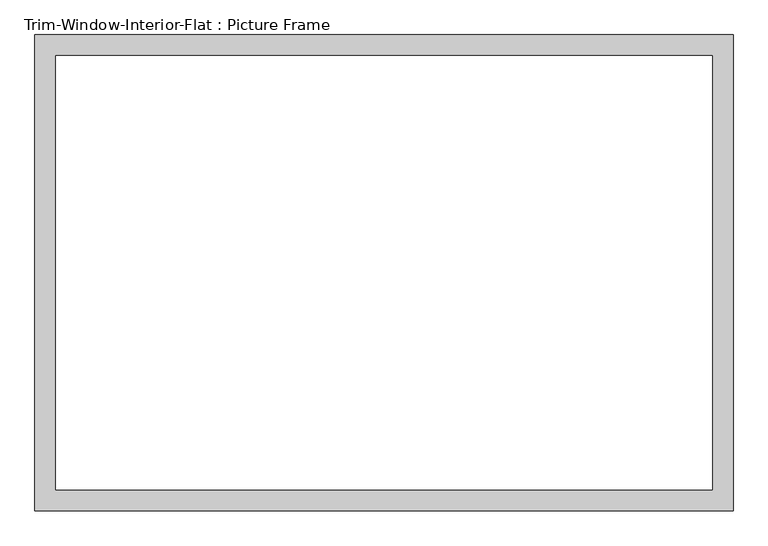
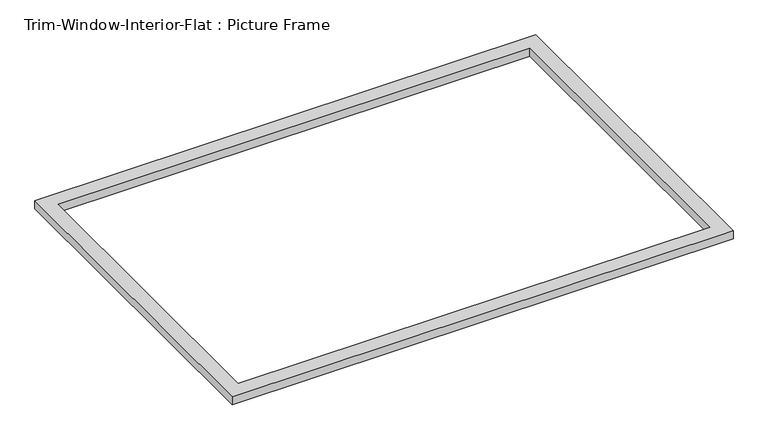
"""IFC4 building model written with IfcOpenShell, lengths in millimetres: proxy geometry, Trim-Window-Interior-Flat : Picture Frame."""

from ifc_helpers import new_model, si_unit, origin, origin_with_axes, place, context, project, spatial, polyline, outline, extrude, source, transform, mapped, element, save


def trim_window_interior_flat_picture_frame_bbff334a(model_context):
    return source(origin(), model_context, "Body", "SweptSolid", [
        extrude(outline(polyline([(958.85, -44.45), (-958.85, -44.45), (-958.85, 1263.65), (958.85, 1263.65), (958.85, -44.45)]), holes=[polyline([(901.7, 12.7), (901.7, 1206.5), (-901.7, 1206.5), (-901.7, 12.7), (901.7, 12.7)])]), origin_with_axes(), (0.0, 0.0, 1.0), 31.75),
    ])


if __name__ == "__main__":
    model = new_model("IFC4")
    model_context = context("Model", 3, world=origin())
    ifc_project = project(units=[si_unit("LENGTHUNIT", "METRE", prefix="MILLI")], contexts=[model_context])
    site = spatial("IfcSite", under=ifc_project)
    building = spatial("IfcBuilding", under=site)
    placement = place(None, origin())
    trim_window_interior_flat_picture_frame_shape = trim_window_interior_flat_picture_frame_bbff334a(model_context)
    element("IfcBuildingElementProxy", 1, Name="Trim-Window-Interior-Flat : Picture Frame", ObjectType="Trim-Window-Interior-Flat : Picture Frame", at=placement, inside=building, context=model_context, shape_type="MappedRepresentation", body=[
        mapped(trim_window_interior_flat_picture_frame_shape, transform((0.0, 0.0, 0.0), x_axis=(1.0, 0.0, 0.0), y_axis=(0.0, 1.0, 0.0), z_axis=(0.0, 0.0, 1.0))),
    ])
    save(model, "model.ifc")

# Revit data of these elements
# Type "Trim-Window-Interior-Flat : Picture Frame"
#   Trim Thickness_Picture Frame = 0' - 1 1/4"
#   Trim Width = 0' - 2 1/4"
#   Trim Thickness_with Sill = 0' - 0 3/4"
#   Sill Thickness = 0' - 1 1/4"
#   Opening Width [instance default] = 2' - 0"
#   Opening Height [instance default] = 3' - 0"
#   Default Elevation = 4' - 0"
#   Sill = no
#   Picture Frame = yes
#   Trim Material [instance default] = none
# Element 1 (IfcBuildingElementProxy, "Trim-Window-Interior-Flat : Picture Frame")
#   Opening Width = 6' - 0"
#   Opening Height = 4' - 0"
#   Trim Material = Wood - Stained
#   Materials on its faces: "Wood - Stained"
# Materials
#   "Wood - Stained": class "Wood", colour RGB 224 178 126, transparency 0, Cost = 0
